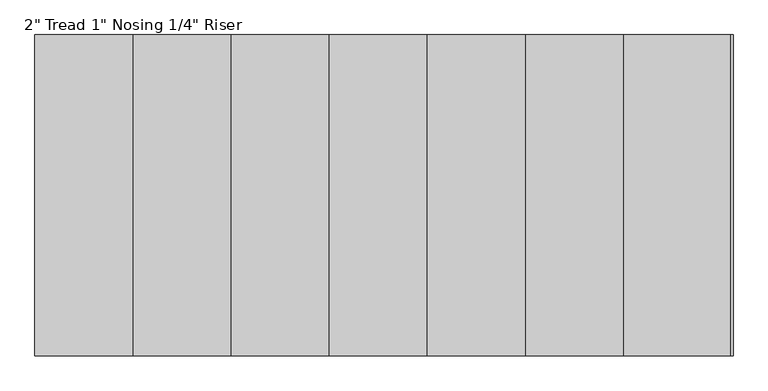
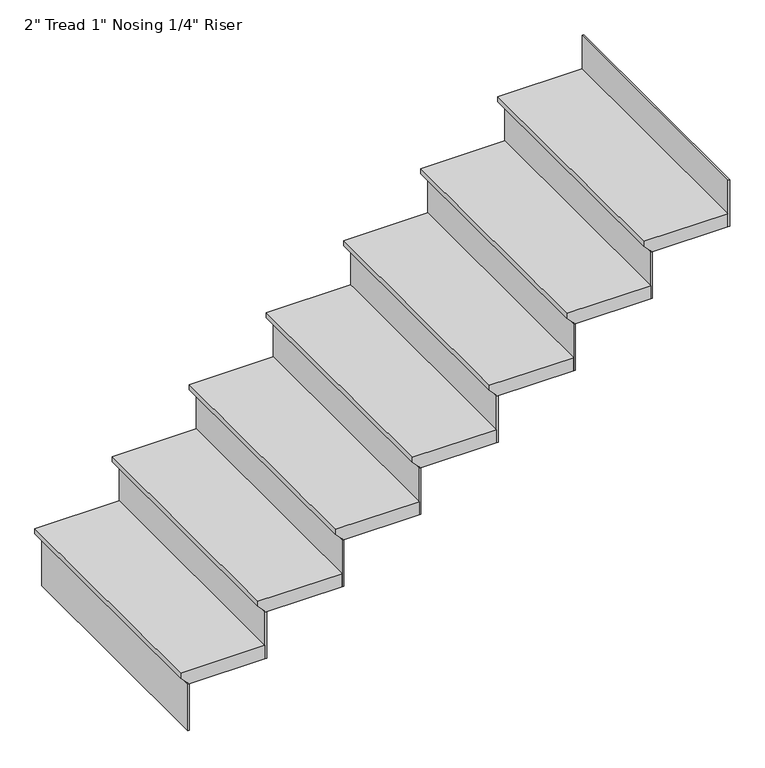
"""IFC4 building model written with IfcOpenShell, lengths in millimetres: stair flight geometry."""

from ifc_helpers import new_model, si_unit, frame, origin, place, context, project, spatial, polyline, outline, extrude, source, transform, mapped, element, save


def stair_flight_d241fc77(model_context):
    return source(origin(), model_context, "Body", "SweptSolid", [
        extrude(outline(polyline([(2565.4, -11753.6120641), (2565.4, -12058.4120641), (2546.35, -12058.4120641), (2520.95, -12033.0120641), (2514.6, -12033.0120641), (2514.6, -11753.6120641), (2565.4, -11753.6120641)])), frame((0.0, -4817.9038196, 0.0), z_axis=(0.0, 1.0, 0.0), x_axis=(0.0, 0.0, 1.0)), (0.0, 0.0, 1.0), 914.4),
        extrude(outline(polyline([(-12026.6620641, -4817.9038196), (-12033.0120641, -4817.9038196), (-12033.0120641, -3903.5038196), (-12026.6620641, -3903.5038196), (-12026.6620641, -4817.9038196)])), frame((0.0, 0.0, 2336.8), z_axis=(0.0, 0.0, 1.0), x_axis=(1.0, 0.0, 0.0)), (0.0, 0.0, 1.0), 177.8),
        extrude(outline(polyline([(-11747.2620641, -4817.9038196), (-11753.6120641, -4817.9038196), (-11753.6120641, -3903.5038196), (-11747.2620641, -3903.5038196), (-11747.2620641, -4817.9038196)])), frame((0.0, 0.0, 2514.6), z_axis=(0.0, 0.0, 1.0), x_axis=(1.0, 0.0, 0.0)), (0.0, 0.0, 1.0), 177.8),
        extrude(outline(polyline([(2743.2, -11474.2120641), (2743.2, -11779.0120641), (2724.15, -11779.0120641), (2698.75, -11753.6120641), (2692.4, -11753.6120641), (2692.4, -11474.2120641), (2743.2, -11474.2120641)])), frame((0.0, -4817.9038196, 0.0), z_axis=(0.0, 1.0, 0.0), x_axis=(0.0, 0.0, 1.0)), (0.0, 0.0, 1.0), 914.4),
        extrude(outline(polyline([(-11467.8620641, -4817.9038196), (-11474.2120641, -4817.9038196), (-11474.2120641, -3903.5038196), (-11467.8620641, -3903.5038196), (-11467.8620641, -4817.9038196)])), frame((0.0, 0.0, 2692.4), z_axis=(0.0, 0.0, 1.0), x_axis=(1.0, 0.0, 0.0)), (0.0, 0.0, 1.0), 177.8),
        extrude(outline(polyline([(2921.0, -11194.8120641), (2921.0, -11499.6120641), (2901.95, -11499.6120641), (2876.55, -11474.2120641), (2870.2, -11474.2120641), (2870.2, -11194.8120641), (2921.0, -11194.8120641)])), frame((0.0, -4817.9038196, 0.0), z_axis=(0.0, 1.0, 0.0), x_axis=(0.0, 0.0, 1.0)), (0.0, 0.0, 1.0), 914.4),
        extrude(outline(polyline([(-11188.4620641, -4817.9038196), (-11194.8120641, -4817.9038196), (-11194.8120641, -3903.5038196), (-11188.4620641, -3903.5038196), (-11188.4620641, -4817.9038196)])), frame((0.0, 0.0, 2870.2), z_axis=(0.0, 0.0, 1.0), x_axis=(1.0, 0.0, 0.0)), (0.0, 0.0, 1.0), 177.8),
        extrude(outline(polyline([(3098.8, -10915.4120641), (3098.8, -11220.2120641), (3079.75, -11220.2120641), (3054.35, -11194.8120641), (3048.0, -11194.8120641), (3048.0, -10915.4120641), (3098.8, -10915.4120641)])), frame((0.0, -4817.9038196, 0.0), z_axis=(0.0, 1.0, 0.0), x_axis=(0.0, 0.0, 1.0)), (0.0, 0.0, 1.0), 914.4),
        extrude(outline(polyline([(-10909.0620641, -4817.9038196), (-10915.4120641, -4817.9038196), (-10915.4120641, -3903.5038196), (-10909.0620641, -3903.5038196), (-10909.0620641, -4817.9038196)])), frame((0.0, 0.0, 3048.0), z_axis=(0.0, 0.0, 1.0), x_axis=(1.0, 0.0, 0.0)), (0.0, 0.0, 1.0), 177.8),
        extrude(outline(polyline([(3276.6, -10636.0120641), (3276.6, -10940.8120641), (3257.55, -10940.8120641), (3232.15, -10915.4120641), (3225.8, -10915.4120641), (3225.8, -10636.0120641), (3276.6, -10636.0120641)])), frame((0.0, -4817.9038196, 0.0), z_axis=(0.0, 1.0, 0.0), x_axis=(0.0, 0.0, 1.0)), (0.0, 0.0, 1.0), 914.4),
        extrude(outline(polyline([(-10629.6620641, -4817.9038196), (-10636.0120641, -4817.9038196), (-10636.0120641, -3903.5038196), (-10629.6620641, -3903.5038196), (-10629.6620641, -4817.9038196)])), frame((0.0, 0.0, 3225.8), z_axis=(0.0, 0.0, 1.0), x_axis=(1.0, 0.0, 0.0)), (0.0, 0.0, 1.0), 177.8),
        extrude(outline(polyline([(3454.4, -10356.6120641), (3454.4, -10661.4120641), (3435.35, -10661.4120641), (3409.95, -10636.0120641), (3403.6, -10636.0120641), (3403.6, -10356.6120641), (3454.4, -10356.6120641)])), frame((0.0, -4817.9038196, 0.0), z_axis=(0.0, 1.0, 0.0), x_axis=(0.0, 0.0, 1.0)), (0.0, 0.0, 1.0), 914.4),
        extrude(outline(polyline([(-10350.2620641, -4817.9038196), (-10356.6120641, -4817.9038196), (-10356.6120641, -3903.5038196), (-10350.2620641, -3903.5038196), (-10350.2620641, -4817.9038196)])), frame((0.0, 0.0, 3403.6), z_axis=(0.0, 0.0, 1.0), x_axis=(1.0, 0.0, 0.0)), (0.0, 0.0, 1.0), 177.8),
        extrude(outline(polyline([(-10070.8620641, -4817.9038196), (-10077.2120641, -4817.9038196), (-10077.2120641, -3903.5038196), (-10070.8620641, -3903.5038196), (-10070.8620641, -4817.9038196)])), frame((0.0, 0.0, 3581.4), z_axis=(0.0, 0.0, 1.0), x_axis=(1.0, 0.0, 0.0)), (0.0, 0.0, 1.0), 177.8),
        extrude(outline(polyline([(3632.2, -10077.2120641), (3632.2, -10382.0120641), (3613.15, -10382.0120641), (3587.75, -10356.6120641), (3581.4, -10356.6120641), (3581.4, -10077.2120641), (3632.2, -10077.2120641)])), frame((0.0, -4817.9038196, 0.0), z_axis=(0.0, 1.0, 0.0), x_axis=(0.0, 0.0, 1.0)), (0.0, 0.0, 1.0), 914.4),
    ])


if __name__ == "__main__":
    model = new_model("IFC4")
    model_context = context("Model", 3, world=origin())
    ifc_project = project(units=[si_unit("LENGTHUNIT", "METRE", prefix="MILLI")], contexts=[model_context])
    site = spatial("IfcSite", under=ifc_project)
    building = spatial("IfcBuilding", under=site)
    placement = place(None, origin())
    stair_flight_shape = stair_flight_d241fc77(model_context)
    element("IfcStairFlight", 1, ObjectType="2\" Tread 1\" Nosing 1/4\" Riser", at=placement, inside=building, context=model_context, shape_type="MappedRepresentation", body=[
        mapped(stair_flight_shape, transform((0.0, 0.0, 0.0), x_axis=(1.0, 0.0, 0.0), y_axis=(0.0, 1.0, 0.0), z_axis=(0.0, 0.0, 1.0))),
    ])
    save(model, "model.ifc")
